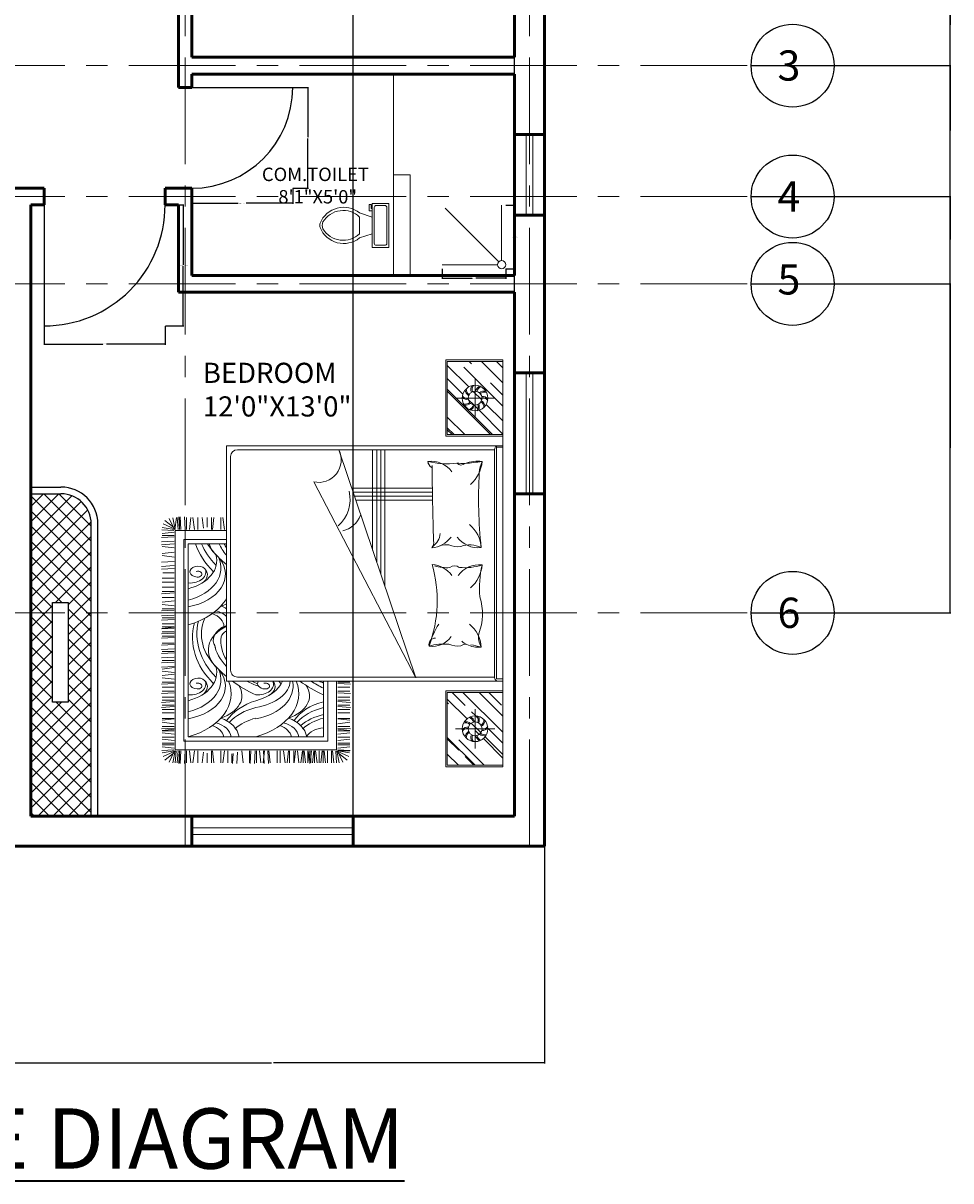
# Model space of a CAD drawing. Units: inches. Extents: x 10696 to 11614, y 5787 to 6498.
# Tile 7 of 9: x 11338 to 11614, y 5787 to 6132. Entities that reach past the tile are written whole.
import ezdxf

# ---------------------------------------------------------------- set-up
doc = ezdxf.new("R2010")
doc.units = ezdxf.units.IN
doc.linetypes.add('CENTER', pattern=[50.8, 31.75, -6.35, 6.35, -6.35])
for name, color, linetype, lineweight in [('A-ANNO-DIMS', 2, 'Continuous', 18), ('A-ANNO-TITL', 7, 'Continuous', 35), ('A-AREA-IDEN', 7, 'Continuous', 25), ('A-DOOR', 3, 'Continuous', 25), ('A-FLOR-CASE', 32, 'Continuous', 25), ('A-FLOR-CASE-PATT', 252, 'Continuous', 13), ('A-FLOR-FIXT', 9, 'Continuous', 20), ('A-FURN', 8, 'Continuous', 18), ('A-GLAZ', 4, 'Continuous', 20), ('A-GRID', 1, 'CENTER', 18), ('A-GRID-IDEN', 1, 'Continuous', 25), ('A-WALL', 7, 'Continuous', 50)]:
    doc.layers.add(name, color=color, linetype=linetype, lineweight=lineweight)
doc.styles.get("Standard").update_dxf_attribs({"font": 'arial.ttf'})
doc.dimstyles.get("Standard").update_dxf_attribs({"dimtxt": 0.18, "dimasz": 0.18, "dimexe": 0.18, "dimexo": 0.0625, "dimgap": 0.09, "dimtad": 0, "dimtih": 1, "dimtoh": 1, "dimdec": 4, "dimzin": 0, "dimdsep": 46, "dimtxsty": 'Standard', "dimcen": 0.09, "dimadec": 0, "dimazin": 0, "dimtfac": 1, "dimtdec": 4, "dimtofl": 0, "dimtmove": 0, "dimatfit": 3, "dimfxl": 1, "dimtolj": 1, "dimtzin": 0, "dimarcsym": 0})

# ---------------------------------------------------------------- blocks, each defined once
blk = doc.blocks.new('A$C64B41DC1')
for p, q in [((0, 2.5079), (2.9903, 2.5079)), ((0, 2.0879), (0, 2.5079)), ((0.012, 2.4618), (0.0581, 2.5079)), ((0.012, 2.3515), (0.1684, 2.5079)), ((0.012, 2.0999), (0.012, 2.5079)), ((0.0543, 2.2213), (0.3409, 2.5079)), ((0.1689, 2.4179), (0.2589, 2.5079)), ((0.3265, 2.386), (0.4484, 2.5079)), ((0.3699, 2.3332), (0.5445, 2.5079)), ((0.548, 2.5079), (0.548, 2.0999)), ((0.56, 2.5079), (0.56, 2.0879)), ((0.6301, 2.5079), (0.6301, 0.4779)), ((0.6401, 2.461), (0.6401, 2.5079)), ((0.6401, 2.5079), (2.344, 2.5079)), ((2.344, 2.5079), (2.3601, 2.5079)), ((2.344, 2.5079), (2.344, 2.461)), ((2.3601, 2.5079), (2.3601, 2.4761)), ((2.3601, 0.4779), (2.3601, 2.5079)), ((2.4303, 2.5079), (2.4303, 2.0879)), ((2.4423, 2.5079), (2.4423, 2.0999)), ((2.4423, 2.3333), (2.6169, 2.5079)), ((2.4423, 2.2145), (2.7357, 2.5079)), ((2.4423, 2.404), (2.5354, 2.4971)), ((2.705, 2.398), (2.8149, 2.5079)), ((2.7691, 2.3772), (2.8998, 2.5079)), ((2.7819, 2.3646), (2.9252, 2.5079)), ((2.9783, 2.0999), (2.9783, 2.5079)), ((2.9903, 2.0879), (2.9903, 2.5079)), ((0.2157, 2.0999), (0.548, 2.4322)), ((0.2299, 2.0999), (0.548, 2.418)), ((0.2804, 2.1597), (0.2804, 2.4481)), ((2.344, 2.461), (0.6401, 2.461)), ((0.6601, 2.4461), (1.4951, 2.4461)), ((0.6601, 2.4461), (0.6601, 0.5579)), ((1.4951, 2.4461), (0.6697, 2.4461)), ((2.3301, 2.4461), (1.4951, 2.4461)), ((2.3301, 0.5579), (2.3301, 2.4461)), ((2.7099, 2.1597), (2.7099, 2.4481)), ((0.1362, 2.3039), (0.4246, 2.3039)), ((0.2311, 2.2906), (0.2937, 2.3532)), ((0.3405, 2.3039), (0.3605, 2.3238)), ((2.8541, 2.3039), (2.5657, 2.3039)), ((2.5849, 2.2779), (2.6158, 2.3088)), ((2.6158, 2.3088), (2.6313, 2.3243)), ((2.6674, 2.2756), (2.7382, 2.3464)), ((2.7249, 2.3076), (2.7512, 2.3339)), ((2.7746, 2.0999), (2.9783, 2.3036)), ((2.7914, 2.1846), (2.9783, 2.3715)), ((0.012, 2.261), (0.0275, 2.2765)), ((0.0404, 2.0999), (0.1982, 2.2578)), ((0.1365, 2.0999), (0.251, 2.2144)), ((0.2905, 2.2539), (0.3304, 2.2938)), ((0.4194, 2.0999), (0.548, 2.2285)), ((2.4423, 2.1353), (2.5382, 2.2312)), ((2.4918, 2.0999), (2.6366, 2.2447)), ((2.9144, 2.2312), (2.9783, 2.2951)), ((0.4986, 2.0999), (0.548, 2.1493)), ((0.5127, 2.0999), (0.548, 2.1352)), ((2.7831, 2.0999), (2.8678, 2.1846)), ((2.8962, 2.0999), (2.9783, 2.182)), ((0.56, 2.0879), (0, 2.0879)), ((0.548, 2.0999), (0.012, 2.0999)), ((2.4303, 2.0879), (2.9903, 2.0879)), ((2.4423, 2.0999), (2.9783, 2.0999)), ((2.5172, 2.0999), (2.5269, 2.1096)), ((0.9415, 1.9902), (0.9415, 1.3975)), ((0.9715, 1.9906), (0.9715, 1.4076)), ((1.0015, 1.991), (1.0015, 1.4177)), ((1.0315, 1.9916), (1.0315, 1.4279)), ((2.3349, 1.8678), (0.6613, 1.3029)), ((0.8956, 1.1191), (2.3349, 1.8678)), ((1.6636, 1.6412), (0.6601, 1.6412)), ((1.5748, 1.6112), (0.6601, 1.6112)), ((2.3665, 1.295), (2.3665, 1.3839)), ((2.377, 1.295), (2.3822, 1.3891)), ((2.4032, 1.295), (2.4032, 1.3839)), ((2.4346, 1.295), (2.4346, 1.3839)), ((2.4451, 1.295), (2.4503, 1.3891)), ((2.4774, 1.2957), (2.4774, 1.3837)), ((2.5, 1.295), (2.5, 1.3839)), ((2.5105, 1.295), (2.5157, 1.3891)), ((2.5367, 1.295), (2.5367, 1.3839)), ((2.5471, 1.295), (2.5524, 1.3891)), ((2.5681, 1.295), (2.5681, 1.3839)), ((2.5918, 1.295), (2.5918, 1.3839)), ((2.6346, 1.2957), (2.6346, 1.3837)), ((2.6362, 1.2957), (2.6467, 1.3839)), ((2.6729, 1.295), (2.6624, 1.3839)), ((2.6938, 1.295), (2.6938, 1.3839)), ((2.7043, 1.295), (2.7095, 1.3891)), ((2.7127, 1.2957), (2.7232, 1.3839)), ((2.7253, 1.295), (2.7253, 1.3839)), ((2.7494, 1.295), (2.7389, 1.3839)), ((2.7718, 1.295), (2.7718, 1.3839)), ((2.7959, 1.295), (2.7854, 1.3839)), ((2.8146, 1.2957), (2.8146, 1.3837)), ((2.8146, 1.2957), (2.8146, 1.3837)), ((2.8282, 1.295), (2.8282, 1.3839)), ((2.8282, 1.295), (2.8282, 1.3839)), ((2.8523, 1.295), (2.8418, 1.3839)), ((2.8523, 1.295), (2.8418, 1.3839)), ((2.8653, 1.2966), (2.8688, 1.3861)), ((2.8711, 1.2957), (2.8711, 1.3837)), ((2.8711, 1.2957), (2.8875, 1.3822)), ((2.8765, 1.2958), (2.9132, 1.3758)), ((2.8893, 1.3011), (2.9394, 1.3636)), ((2.3601, 1.2873), (2.8639, 1.2873)), ((2.8639, 1.2873), (2.8639, 0.1018)), ((2.8713, 1.2927), (2.954, 1.3315)), ((2.8717, 1.2884), (2.9588, 1.3058)), ((2.8744, 1.2817), (2.9603, 1.2869)), ((2.3601, 1.2233), (2.7999, 1.2233)), ((2.3601, 1.1913), (2.7679, 1.1912)), ((2.7679, 1.1912), (2.7679, 0.1978)), ((2.7999, 1.2233), (2.7999, 0.1658)), ((2.8716, 1.2565), (2.9605, 1.2669)), ((2.8716, 1.2212), (2.9605, 1.2212)), ((2.8716, 1.1947), (2.9605, 1.2052)), ((2.8723, 1.2489), (2.9603, 1.2489)), ((2.8716, 1.181), (2.9605, 1.1705)), ((2.8716, 1.1595), (2.9605, 1.1595)), ((2.8716, 1.133), (2.9605, 1.1435)), ((2.8716, 1.1193), (2.9605, 1.1088)), ((2.8723, 1.1872), (2.9603, 1.1872)), ((2.8723, 1.1255), (2.9603, 1.1255)), ((2.8716, 1.1035), (2.9605, 1.093)), ((2.8716, 1.0965), (2.9605, 1.0965)), ((2.8716, 1.086), (2.9657, 1.0913)), ((2.8716, 1.0756), (2.9605, 1.0756)), ((2.8716, 1.0491), (2.9605, 1.0596)), ((2.8716, 1.0354), (2.9605, 1.0249)), ((2.8723, 1.0858), (2.9605, 1.0753)), ((2.8723, 1.0416), (2.9603, 1.0416)), ((2.8723, 0.9987), (2.9605, 1.0092)), ((2.8723, 0.985), (2.9605, 0.9745)), ((2.8723, 0.9735), (2.9603, 0.9735)), ((2.8723, 0.9408), (2.9603, 0.9408)), ((2.8716, 0.9346), (2.9605, 0.9241)), ((2.8723, 0.8979), (2.9605, 0.9084)), ((2.8723, 0.8726), (2.9603, 0.8726)), ((2.8716, 0.7885), (2.9605, 0.799)), ((2.8716, 0.7818), (2.9657, 0.787)), ((2.8723, 0.8505), (2.9603, 0.8505)), ((2.8716, 0.7503), (2.9657, 0.7556)), ((2.8716, 0.7204), (2.9605, 0.7309)), ((2.8716, 0.6995), (2.9605, 0.6995)), ((2.8716, 0.689), (2.9657, 0.6838)), ((2.8723, 0.7571), (2.9605, 0.7466)), ((2.8716, 0.6576), (2.9657, 0.6523)), ((2.8716, 0.6471), (2.9605, 0.6471)), ((2.8716, 0.5903), (2.9605, 0.6007)), ((2.882, 0.5582), (2.9657, 0.5536)), ((2.8909, 0.5263), (2.9657, 0.5222)), ((2.8928, 0.5169), (2.9605, 0.5169)), ((0.6301, 0.4779), (2.3601, 0.4779)), ((0.7101, 0.5079), (2.2801, 0.5079)), ((1.2465, 0.4625), (1.1576, 0.452)), ((1.2465, 0.4365), (1.1577, 0.4365)), ((1.2542, 0.1018), (1.2542, 0.4779)), ((1.3182, 0.1658), (1.3182, 0.4779)), ((1.3502, 0.1978), (1.3502, 0.4779)), ((2.8716, 0.4877), (2.9603, 0.4877)), ((2.8716, 0.4625), (2.9605, 0.452)), ((2.8716, 0.4365), (2.9603, 0.4365)), ((1.2465, 0.3746), (1.1576, 0.3851)), ((1.2465, 0.3684), (1.1577, 0.3684)), ((2.8716, 0.3746), (2.9605, 0.3851)), ((2.8716, 0.3684), (2.9603, 0.3684)), ((1.2355, 0.3092), (1.1576, 0.3)), ((1.2285, 0.3357), (1.1577, 0.3357)), ((1.2457, 0.2676), (1.1577, 0.2676)), ((2.8723, 0.2676), (2.9603, 0.2676)), ((2.8826, 0.3092), (2.9605, 0.3)), ((2.8896, 0.3357), (2.9603, 0.3357)), ((1.2465, 0.1742), (1.1524, 0.169)), ((1.2457, 0.2423), (1.1576, 0.2319)), ((1.2465, 0.2057), (1.1576, 0.2161)), ((1.2465, 0.1847), (1.1576, 0.1847)), ((2.7679, 0.1978), (1.3502, 0.1978)), ((2.8716, 0.2057), (2.9605, 0.2161)), ((2.8716, 0.1847), (2.9605, 0.1847)), ((2.8716, 0.1742), (2.9657, 0.169)), ((2.8723, 0.2423), (2.9605, 0.2319)), ((1.2465, 0.1428), (1.1524, 0.1376)), ((1.2465, 0.1334), (1.1524, 0.1281)), ((1.2465, 0.1323), (1.1576, 0.1323)), ((1.2465, 0.1323), (1.1576, 0.1323)), ((1.2465, 0.1), (1.1576, 0.1105)), ((1.2465, 0.1229), (1.1588, 0.1168)), ((1.2464, 0.1007), (1.1592, 0.0833)), ((1.2468, 0.0964), (1.1641, 0.0576)), ((1.2288, 0.088), (1.1787, 0.0255)), ((1.2415, 0.0933), (1.2049, 0.0133)), ((1.247, 0.0934), (1.2306, 0.0069)), ((1.2527, 0.0925), (1.2493, 0.003)), ((2.8639, 0.1018), (1.2542, 0.1018)), ((1.2658, 0.0941), (1.2762, 0.0052)), ((1.2899, 0.0941), (1.2899, 0.0052)), ((1.2999, 0.0941), (1.3051, 0)), ((2.7999, 0.1658), (1.3182, 0.1658)), ((1.3313, 0.0941), (1.3365, 0)), ((1.3523, 0.0941), (1.3575, 0)), ((1.3804, 0.0941), (1.3699, 0.0052)), ((1.4119, 0.0934), (1.4223, 0.0052)), ((1.4485, 0.0941), (1.438, 0.0052)), ((1.48, 0.0941), (1.4852, 0)), ((1.5114, 0.0941), (1.5166, 0)), ((1.5323, 0.0941), (1.5376, 0)), ((1.5638, 0.0941), (1.5638, 0.0105)), ((1.6021, 0.0941), (1.6021, 0.0052)), ((1.6336, 0.0941), (1.6336, 0.0052)), ((1.6702, 0.0941), (1.6702, 0.0052)), ((1.7017, 0.0941), (1.7017, 0.0052)), ((1.7122, 0.0941), (1.7174, 0)), ((1.7445, 0.0934), (1.7445, 0.0054)), ((1.7698, 0.0934), (1.7803, 0.0052)), ((1.8065, 0.0941), (1.796, 0.0052)), ((1.8274, 0.0941), (1.8274, 0.0052)), ((1.8379, 0.0941), (1.8431, 0)), ((1.8746, 0.0941), (1.8798, 0)), ((1.8955, 0.0941), (1.8955, 0.0052)), ((1.906, 0.0941), (1.9113, 0)), ((1.9384, 0.0934), (1.9384, 0.0054)), ((1.9609, 0.0941), (1.9609, 0.0052)), ((1.9636, 0.0934), (1.9741, 0.0052)), ((1.9714, 0.0941), (1.9766, 0)), ((1.9976, 0.0941), (1.9976, 0.0052)), ((2.0081, 0.0941), (2.0133, 0)), ((2.029, 0.0941), (2.029, 0.0052)), ((2.0395, 0.0941), (2.0447, 0)), ((2.0797, 0.0941), (2.0797, 0.0052)), ((2.0902, 0.0941), (2.0954, 0)), ((2.1216, 0.0941), (2.1269, 0)), ((2.1412, 0.0941), (2.1412, 0.0052)), ((2.1517, 0.0941), (2.1569, 0)), ((2.1831, 0.0941), (2.1884, 0)), ((2.2093, 0.0941), (2.2093, 0.0052)), ((2.2198, 0.0941), (2.225, 0)), ((2.2512, 0.0941), (2.2565, 0)), ((2.2603, 0.0934), (2.2707, 0.0052)), ((2.2969, 0.0941), (2.2864, 0.0052)), ((2.3089, 0.0934), (2.3193, 0.0052)), ((2.3455, 0.0941), (2.3351, 0.0052)), ((2.3665, 0.0941), (2.3665, 0.0052)), ((2.377, 0.0941), (2.3822, 0)), ((2.4032, 0.0941), (2.4032, 0.0052)), ((2.4346, 0.0941), (2.4346, 0.0052)), ((2.4451, 0.0941), (2.4503, 0)), ((2.4774, 0.0934), (2.4774, 0.0054)), ((2.5, 0.0941), (2.5, 0.0052)), ((2.5105, 0.0941), (2.5157, 0)), ((2.5367, 0.0941), (2.5367, 0.0052)), ((2.5471, 0.0941), (2.5524, 0)), ((2.5681, 0.0941), (2.5681, 0.0052)), ((2.5918, 0.0941), (2.5918, 0.0052)), ((2.6346, 0.0934), (2.6346, 0.0054)), ((2.6362, 0.0934), (2.6467, 0.0052)), ((2.6729, 0.0941), (2.6624, 0.0052)), ((2.6938, 0.0941), (2.6938, 0.0052)), ((2.7043, 0.0941), (2.7095, 0)), ((2.7127, 0.0934), (2.7232, 0.0052)), ((2.7253, 0.0941), (2.7253, 0.0052)), ((2.7494, 0.0941), (2.7389, 0.0052)), ((2.7718, 0.0941), (2.7718, 0.0052)), ((2.7959, 0.0941), (2.7854, 0.0052)), ((2.8146, 0.0934), (2.8146, 0.0054)), ((2.8282, 0.0941), (2.8282, 0.0052)), ((2.8523, 0.0941), (2.8418, 0.0052)), ((2.8653, 0.0925), (2.8688, 0.003)), ((2.8711, 0.0934), (2.8875, 0.0069)), ((2.8713, 0.0964), (2.954, 0.0576)), ((2.8716, 0.1428), (2.9657, 0.1376)), ((2.8716, 0.1334), (2.9657, 0.1281)), ((2.8716, 0.1323), (2.9605, 0.1323)), ((2.8716, 0.1229), (2.9593, 0.1168)), ((2.8717, 0.1007), (2.9588, 0.0833)), ((2.8744, 0.1074), (2.9603, 0.1022)), ((2.8765, 0.0933), (2.9132, 0.0133)), ((2.8893, 0.088), (2.9394, 0.0255))]:
    blk.add_line(p, q)
at = {"ltscale": 10}
for p, q in [((1.4859, 1.5812), (0.6601, 1.5812)), ((1.397, 1.5512), (0.6601, 1.5512))]:
    blk.add_line(p, q, dxfattribs=at)
for centre, radius in [((0.2804, 2.3039), 0.0942), ((2.7099, 2.3039), 0.0942), ((0.2804, 2.3039), 0.051), ((2.7099, 2.3039), 0.051)]:
    blk.add_circle(centre, radius)
for centre, radius, start, end in [((0.6601, 2.4761), 0.03, 180, 270), ((2.3301, 2.4761), 0.03, 270, 0), ((0.2887, 2.3745), 0.0605, 172.17003, 218.48975), ((0.2828, 2.3731), 0.0462, 160.30017, 220.53802), ((0.3286, 2.3561), 0.0605, 136.17003, 182.48975), ((0.3231, 2.3585), 0.0462, 124.30017, 184.53802), ((2.6672, 2.3585), 0.0462, 355.46198, 55.69983), ((2.6617, 2.3561), 0.0605, 357.51025, 43.82997), ((2.7075, 2.3731), 0.0462, 319.46198, 19.69983), ((2.7016, 2.3745), 0.0605, 321.51025, 7.82997), ((0.2457, 2.3659), 0.0605, 208.17003, 254.48975), ((0.2417, 2.3614), 0.0462, 196.30017, 256.53802), ((0.3501, 2.3178), 0.0605, 100.17003, 146.48975), ((0.347, 2.323), 0.0462, 88.30017, 148.53802), ((0.3449, 2.2742), 0.0605, 64.17003, 110.48975), ((0.3455, 2.2802), 0.0462, 52.30017, 112.53802), ((0.3151, 2.2419), 0.0605, 28.17003, 74.48975), ((1.0526, 2.3302), 0.3085, 175.30484, 198.69419), ((-0.8702, 2.0941), 1.6364, 4.80985, 9.18918), ((0.8579, 2.6278), 0.2948, 247.51785, 264.26696), ((0.728, 2.111), 0.245, 40.4189, 85.9871), ((1.0164, 5.7096), 3.3803, 266.81337, 276.16021), ((1.3963, 2.1044), 0.245, 94.0129, 139.5811), ((1.1858, 2.3288), 0.1943, 306.5711, 5.88998), ((1.5348, 2.2652), 0.1767, 151.77364, 201.69827), ((1.6986, 2.3355), 0.1943, 174.11002, 233.4289), ((1.1481, 2.2311), 0.3783, 353.49469, 19.18669), ((1.6871, 3.192), 0.8561, 257.74383, 273.62843), ((1.4882, 2.111), 0.245, 40.4189, 85.9871), ((1.8674, 1.9709), 0.3878, 68.20259, 108.9817), ((2.1269, 2.1044), 0.245, 94.0129, 139.5811), ((2.0342, 2.4856), 0.1563, 261.59582, 298.90918), ((1.9165, 2.3288), 0.1943, 333.73715, 5.88998), ((2.6058, 2.2028), 0.517, 163.60457, 172.3273), ((2.6448, 2.2802), 0.0462, 67.46198, 127.69983), ((2.6454, 2.2742), 0.0605, 69.51025, 115.82997), ((2.6752, 2.2419), 0.0605, 105.51025, 151.82997), ((2.6433, 2.323), 0.0462, 31.46198, 91.69983), ((2.6402, 2.3178), 0.0605, 33.51025, 79.82997), ((2.7486, 2.3614), 0.0462, 283.46198, 343.69983), ((2.7446, 2.3659), 0.0605, 285.51025, 331.82997), ((0.2153, 2.3276), 0.0462, 232.30017, 292.53802), ((0.2158, 2.3336), 0.0605, 244.17003, 290.48975), ((0.2138, 2.2848), 0.0462, 268.30017, 328.53802), ((0.2107, 2.29), 0.0605, 280.17003, 326.48975), ((0.2377, 2.2493), 0.0462, 304.30017, 4.53802), ((0.2322, 2.2517), 0.0605, 316.17003, 2.48975), ((0.2779, 2.2347), 0.0462, 340.30017, 40.53802), ((0.272, 2.2333), 0.0605, 352.17003, 38.48975), ((0.3191, 2.2464), 0.0462, 16.30017, 76.53802), ((0.7274, 2.2013), 0.0446, 314.4736, 42.17134), ((-1.6008, 2.277), 2.3618, 357.39054, 358.88764), ((1.9165, 2.3288), 0.1943, 320.94042, 333.73715), ((2.1347, 2.2313), 0.0459, 165.35061, 223.26844), ((2.6712, 2.2464), 0.0462, 103.46198, 163.69983), ((2.7182, 2.2333), 0.0605, 141.51025, 187.82997), ((2.7123, 2.2347), 0.0462, 139.46198, 199.69983), ((2.7581, 2.2517), 0.0605, 177.51025, 223.82997), ((2.7526, 2.2493), 0.0462, 175.46198, 235.69983), ((2.7796, 2.29), 0.0605, 213.51025, 259.82997), ((2.7765, 2.2848), 0.0462, 211.46198, 271.69983), ((2.7744, 2.3336), 0.0605, 249.51025, 295.82997), ((2.775, 2.3276), 0.0462, 247.46198, 307.69983), ((0.9385, 1.978), 0.1943, 126.5711, 185.88998), ((0.2688, 2.0945), 0.4956, 344.0243, 8.70709), ((1.1858, 1.9714), 0.1943, 4.31813, 53.4289), ((1.204, 2.1778), 0.1681, 337.01697, 7.53676), ((1.7059, 1.9714), 0.204, 127.11975, 175.09005), ((1.5671, 2.1546), 0.0547, 142.08329, 220.902), ((1.9394, 1.991), 0.1651, 351.26213, 55.75721), ((1.9346, 2.1778), 0.1681, 337.01697, 7.53676), ((1.2687, 1.9248), 0.1223, 33.62799, 86.47438), ((1.5415, 2.0969), 0.1834, 175.22328, 196.23004), ((1.1965, 2.0983), 0.3299, 343.79543, 3.55541), ((2.4617, 2.0719), 0.3745, 173.82958, 196.4356), ((0.7417, 2.0149), 0.057, 273.47085, 328.54118), ((0.728, 2.2025), 0.245, 274.0129, 278.34166), ((0.7246, 18.8439), 16.8552, 270.17399, 272.05214), ((1.3401, 1.9404), 0.0603, 49.09906, 101.37023), ((1.7676, 1.0629), 0.9631, 69.65065, 105.96307), ((2.2748, 2.5795), 0.6373, 238.34989, 254.31375), ((2.0911, 2.0123), 0.0478, 179.77267, 283.80184), ((1.0747, 1.2871), 0.1871, 14.1863, 69.12121), ((1.0274, 1.1334), 0.2527, 40.62904, 104.37123), ((0.7347, 1.1553), 0.1649, 347.31088, 116.44537), ((0.7101, 0.5579), 0.05, 180, 270), ((2.2801, 0.5579), 0.05, 270, 0)]:
    blk.add_arc(centre, radius, start, end)
for centre, major_axis, ratio, start_param, end_param in [((1.9938, 1.6262), (0, -0.7531), 0.68, 0.797284, 0.954936), ((2.0643, 1.466), (0, -0.5322), 0.68, 7.239912, 7.311536), ((1.9052, 1.7397), (0, -0.9842), 0.68, 0.74745, 0.979724), ((2.7455, 1.3081), (0, 0.3614), 0.68, 1.900046, 2.742661), ((2.7868, 1.3081), (0, 0.3614), 0.68, 1.900046, 2.614747), ((2.8372, 1.3081), (0, 0.3614), 0.68, 1.900046, 2.479658), ((2.8607, 1.3211), (0, 0.3614), 0.68, 1.938265, 2.479658), ((2.8057, 1.2079), (0, -0.1524), 0.68, 4.821745, 5.895886), ((2.4665, 0.8216), (0, -0.2664), 0.68, 2.006169, 3.565187), ((2.4513, 0.5069), (0, 0.502), 0.68, 5.095327, 6.553458), ((2.7862, 0.8069), (0, -0.2615), 0.68, 3.244645, 4.205018), ((2.396, 0.6032), (0, 0.3641), 0.68, -1.3172, 0.145284), ((2.3507, 0.5642), (0.0073, 0.3819), 0.56205, -1.21172, -0.009991), ((2.7784, 0.8289), (0, -0.1802), 0.68, 3.227058, 4.318474), ((2.7821, 0.7971), (0, -0.1589), 0.68, 3.272942, 4.229533), ((2.2964, 0.5771), (0, -0.3263), 0.68, 1.938944, 2.850232), ((2.0403, 1.6015), (0, -0.8763), 0.68, 6.849801, 6.887077), ((2.4005, 0.7132), (0, -0.1214), 0.68, 2.284368, 3.652258), ((2.3834, 0.7081), (0, 0.1147), 0.68, 4.593909, 6.585576), ((2.3961, 0.7628), (0, -0.0317), 0.68, 1.462497, 5.046281), ((2.3774, 0.7653), (0, -0.0593), 0.68, 5.841311, 7.755362), ((1.9938, 1.1295), (-0.0678, 0.7439), 0.610498, 3.917146, 4.063997), ((2.0643, 0.9693), (0, -0.5322), 0.68, 7.239912, 7.336618), ((1.9052, 1.243), (0, -0.9842), 0.68, 0.74745, 0.979724), ((2.7455, 0.8114), (-0.0599, 0.3735), 0.695517, 1.775813, 2.548612), ((2.7868, 0.8114), (0, 0.3614), 0.68, 1.900046, 2.614747), ((2.8607, 0.8243), (0, 0.3614), 0.68, 1.938265, 2.479658), ((2.4665, 0.3249), (0, -0.2664), 0.68, 2.006169, 3.565187), ((2.4513, 0.0102), (0, 0.502), 0.68, 5.095327, 6.553458), ((2.7862, 0.3102), (0, -0.2615), 0.68, 3.244645, 4.205018), ((2.7784, 0.3322), (0, -0.1802), 0.68, 3.227058, 4.318474), ((1.242, 0.9693), (0, -0.5322), 0.68, 6.586764, 6.677612), ((1.1714, 1.1295), (-0.1157, 0.7241), 0.59432, 3.291697, 3.50733), ((1.474, 0.0804), (0, -0.3263), 0.68, 1.938944, 3.339184), ((1.0828, 1.243), (0, -0.9842), 0.68, 0.565948, 0.680366), ((1.5283, 0.0674), (0, -0.3703), 0.68, 1.930561, 3.464283), ((1.5736, 0.1065), (0, 0.3641), 0.68, -1.3172, 0.476403), ((1.6289, 0.0102), (0, 0.502), 0.68, 6.655152, 6.661293), ((1.6289, 0.0102), (0, 0.502), 0.68, 5.095327, 5.911219), ((1.6442, 0.3249), (0, -0.2664), 0.68, 2.006169, 2.182797), ((1.9638, 0.3102), (0, -0.2615), 0.68, 4.015924, 4.205018), ((1.956, 0.3322), (0, -0.1802), 0.68, 3.770744, 4.318474), ((1.9597, 0.3004), (0, -0.1589), 0.68, 3.14258, 4.229533), ((2.0606, 0.5616), (0, -0.1803), 0.68, 5.194792, 5.929328), ((2.0606, 0.5616), (0, -0.1803), 0.68, 5.194792, 6.723255), ((2.1315, 0.6603), (0, -0.3155), 0.68, 5.328638, 6.949396), ((2.0549, 0.5656), (0, -0.1303), 0.68, 5.450951, 6.054641), ((2.0643, 0.9693), (0, -0.5322), 0.68, 6.20013, 6.677612), ((1.9938, 1.1295), (-0.0678, 0.7439), 0.610498, 3.199135, 3.592282), ((2.2964, 0.0804), (0, -0.3263), 0.68, 1.938944, 3.339184), ((1.9052, 1.243), (0, -0.9842), 0.68, 0.565948, 0.680366), ((2.3507, 0.0674), (0, -0.3703), 0.68, 1.930561, 3.464283), ((2.396, 0.1065), (0, 0.3641), 0.68, -1.3172, 0.476403), ((2.4513, 0.0102), (0, 0.502), 0.68, 6.655152, 6.661293), ((2.7821, 0.3004), (0, -0.1589), 0.68, 3.272942, 4.229533), ((1.1933, 0.9181), (0, -0.624), 0.68, 0.378672, 0.625379), ((1.3091, 0.6603), (0, -0.3155), 0.68, 6.475719, 6.949396), ((1.1911, 1.1066), (0, 0.8458), 0.68, 3.421828, 3.728616), ((1.2179, 1.1047), (0, -0.8763), 0.68, 6.507006, 6.887077), ((1.5781, 0.2165), (0, -0.1214), 0.68, 2.284368, 3.726131), ((2.0157, 0.9181), (0, -0.624), 0.68, -0.280078, 0.625379), ((2.0135, 1.1066), (0, 0.8458), 0.68, 2.978727, 3.728616), ((2.0403, 1.1047), (0, -0.8763), 0.68, 6.099302, 6.887077), ((2.4005, 0.2165), (0, -0.1214), 0.68, 2.284368, 3.726131), ((1.555, 0.2685), (0, -0.0593), 0.68, 3.732151, 7.755362), ((1.561, 0.2114), (0, 0.1147), 0.68, 4.593909, 6.647252), ((1.5737, 0.2661), (0, -0.0317), 0.68, 1.462497, 5.046281), ((2.3774, 0.2685), (0, -0.0593), 0.68, 3.732151, 7.755362), ((2.3834, 0.2114), (0, 0.1147), 0.68, 4.593909, 6.647252), ((2.3961, 0.2661), (0, -0.0317), 0.68, 1.462497, 5.046281)]:
    blk.add_ellipse(centre, major_axis=major_axis, ratio=ratio, start_param=start_param, end_param=end_param)
blk = doc.blocks.new('*U10')
for p, q in [((9.5, -6), (9.5, -2)), ((-10, -8.5), (-8, -8.5)), ((-10, -9.5), (-10, -8.5)), ((-7, -9.5), (-10, -9.5)), ((-8, -8.5), (-8, -8)), ((-7, -8), (-7, -9.5)), ((-4, -8), (-6, -14)), ((4, -8), (6, -14)), ((4, -14), (-4, -14))]:
    blk.add_line(p, q)
blk.add_lwpolyline([(10.5, -8), (10.5, 0), (-10.5, 0), (-10.5, -8)], close=True)
for points in [[(-9.5, -2), (-9.5, -6)], [(8.5, -1), (-8.5, -1)], [(-8.5, -7), (8.5, -7)]]:
    blk.add_lwpolyline(points)
for centre, radius, start, end in [((-8.62, -1.88), 0.884, 81.8699, 188.1301), ((8.62, -1.88), 0.884, 351.8699, 98.1301), ((-8.62, -6.12), 0.884, 171.8699, 278.1301), ((8.62, -6.12), 0.884, 261.8699, 8.1301), ((3.52, -21.58), 12.17, 141.4691, 247.9714), ((4.2, -21.82), 11.33, 136.3677, 238.9468), ((-3.52, -21.58), 12.17, 292.0284, 38.5307), ((-4.2, -21.82), 11.33, 301.053, 43.6321), ((0, -27.88), 4, 245.7318, 294.2682), ((0, -29), 4, 254.8605, 285.1395)]:
    blk.add_arc(centre, radius, start, end)
blk = doc.blocks.new('DOOR-SINGLE-30')
blk.add_line((0, 30), (30, 30))
blk.add_arc((0, 30), 30, 270, 0)
blk = doc.blocks.new('DOOR-SINGLE-36-BEDROOM')
blk.add_line((0, 36), (0, 0))
blk.add_arc((0.1, 35.9), 35.9, 269.8411, 0.1589)
blk = doc.blocks.new('WIN-GLAZ-24')
for p, q in [((0, 24), (0, 0)), ((2, 24), (2, 0))]:
    blk.add_line(p, q)
blk = doc.blocks.new('WIN-GLAZ-36')
for p, q in [((0, 0), (0, 36)), ((2, 0), (2, 36))]:
    blk.add_line(p, q)
blk = doc.blocks.new('WIN-GLAZ-48')
for p, q in [((0, 48), (0, 0)), ((2, 48), (2, 0))]:
    blk.add_line(p, q)
blk = doc.blocks.new('SHOWER-SCREEN')
for p, q in [((0, 0), (0, 60)), ((0, 30), (5, 30)), ((5, 0), (5, 30))]:
    blk.add_line(p, q)
blk = doc.blocks.new('SHOWER-DRAIN')
for p, q in [((16.81, 2.05), (0.86, 18)), ((17.68, 2.42), (17.68, 18.95)), ((16.47, 1.21), (0, 1.21))]:
    blk.add_line(p, q)
blk.add_circle((17.68, 1.21), 1.21)
blk = doc.blocks.new('*D44')
at = {"layer": 'A-ANNO-DIMS', "color": 0, "lineweight": -2, "transparency": 16777216}
for p, q in [((11387.77, 6083.01), (11387.77, 6078.39)), ((11417.77, 6083.01), (11417.77, 6078.39)), ((11387.95, 6078.57), (11401.58, 6078.57)), ((11417.59, 6078.57), (11403.96, 6078.57))]:
    blk.add_line(p, q, dxfattribs=at)
at = {"layer": 'A-ANNO-DIMS', "color": 0, "transparency": 16777216}
for points in [[(11387.95, 6078.6), (11387.95, 6078.54), (11387.77, 6078.57)], [(11417.59, 6078.6), (11417.59, 6078.54), (11417.77, 6078.57)]]:
    blk.add_solid(points, dxfattribs=at)
at = {"layer": 'Defpoints', "color": 0, "transparency": 16777216}
for p in [(11387.77, 6083.07), (11417.77, 6083.07), (11417.77, 6078.57)]:
    blk.add_point(p, dxfattribs=at)
at = {"layer": 'A-ANNO-DIMS', "color": 0, "transparency": 16777216, "insert": (11402.77, 6078.57), "char_height": 0.18, "attachment_point": 5}
blk.add_mtext('\\A1;WC DOOR 30 TYP.', dxfattribs=at)
blk = doc.blocks.new('*D45')
at = {"layer": 'A-ANNO-DIMS', "color": 0, "lineweight": -2, "transparency": 16777216}
for p, q in [((11417.83, 6113.07), (11422.45, 6113.07)), ((11422.27, 6112.89), (11422.27, 6098.25)), ((11422.27, 6083.25), (11422.27, 6097.89)), ((11417.83, 6083.07), (11422.45, 6083.07))]:
    blk.add_line(p, q, dxfattribs=at)
at = {"layer": 'A-ANNO-DIMS', "color": 0, "transparency": 16777216}
for points in [[(11422.24, 6112.89), (11422.3, 6112.89), (11422.27, 6113.07)], [(11422.24, 6083.25), (11422.3, 6083.25), (11422.27, 6083.07)]]:
    blk.add_solid(points, dxfattribs=at)
at = {"layer": 'Defpoints', "color": 0, "transparency": 16777216}
for p in [(11417.77, 6113.07), (11422.27, 6113.07), (11417.77, 6083.07)]:
    blk.add_point(p, dxfattribs=at)
at = {"layer": 'A-ANNO-DIMS', "color": 0, "transparency": 16777216, "insert": (11422.27, 6098.07), "char_height": 0.18, "attachment_point": 5}
blk.add_mtext('\\A1;30 TYP.', dxfattribs=at)
blk = doc.blocks.new('*D46')
at = {"layer": 'A-ANNO-DIMS', "color": 0, "lineweight": -2, "transparency": 16777216}
for p, q in [((11379.86, 6078.07), (11385.38, 6078.07)), ((11385.2, 6077.89), (11385.2, 6060.24)), ((11385.2, 6042.22), (11385.2, 6059.87)), ((11379.86, 6042.04), (11385.38, 6042.04))]:
    blk.add_line(p, q, dxfattribs=at)
at = {"layer": 'A-ANNO-DIMS', "color": 0, "transparency": 16777216}
for points in [[(11385.17, 6077.89), (11385.23, 6077.89), (11385.2, 6078.07)], [(11385.17, 6042.22), (11385.23, 6042.22), (11385.2, 6042.04)]]:
    blk.add_solid(points, dxfattribs=at)
at = {"layer": 'Defpoints', "color": 0, "transparency": 16777216}
for p in [(11379.79, 6078.07), (11385.2, 6078.07), (11379.79, 6042.04)]:
    blk.add_point(p, dxfattribs=at)
at = {"layer": 'A-ANNO-DIMS', "color": 0, "transparency": 16777216, "insert": (11385.2, 6060.06), "char_height": 0.18, "attachment_point": 5}
blk.add_mtext('\\A1;BEDROOM DOOR 36 TYP.', dxfattribs=at)
blk = doc.blocks.new('*D47')
at = {"layer": 'A-ANNO-DIMS', "color": 0, "lineweight": -2, "transparency": 16777216}
for p, q in [((11343.77, 6041.98), (11343.77, 6036.46)), ((11379.79, 6041.98), (11379.79, 6036.46)), ((11343.95, 6036.64), (11361.25, 6036.64)), ((11379.61, 6036.64), (11362.31, 6036.64))]:
    blk.add_line(p, q, dxfattribs=at)
at = {"layer": 'A-ANNO-DIMS', "color": 0, "transparency": 16777216}
for points in [[(11343.95, 6036.67), (11343.95, 6036.61), (11343.77, 6036.64)], [(11379.61, 6036.67), (11379.61, 6036.61), (11379.79, 6036.64)]]:
    blk.add_solid(points, dxfattribs=at)
at = {"layer": 'Defpoints', "color": 0, "transparency": 16777216}
for p in [(11343.77, 6042.04), (11379.79, 6042.04), (11379.79, 6036.64)]:
    blk.add_point(p, dxfattribs=at)
at = {"layer": 'A-ANNO-DIMS', "color": 0, "transparency": 16777216, "insert": (11361.78, 6036.64), "char_height": 0.18, "attachment_point": 5}
blk.add_mtext('\\A1;36 TYP.', dxfattribs=at)
blk = doc.blocks.new('*D62')
at = {"layer": 'A-ANNO-DIMS', "color": 0, "lineweight": -2, "transparency": 16777216}
for p, q in [((11481.25, 6078.02), (11484.21, 6078.02)), ((11484.03, 6077.84), (11484.03, 6068.73)), ((11484.03, 6059.25), (11484.03, 6068.37)), ((11481.25, 6059.07), (11484.21, 6059.07))]:
    blk.add_line(p, q, dxfattribs=at)
at = {"layer": 'A-ANNO-DIMS', "color": 0, "transparency": 16777216}
for points in [[(11484, 6077.84), (11484.06, 6077.84), (11484.03, 6078.02)], [(11484, 6059.25), (11484.06, 6059.25), (11484.03, 6059.07)]]:
    blk.add_solid(points, dxfattribs=at)
at = {"layer": 'Defpoints', "color": 0, "transparency": 16777216}
for p in [(11481.19, 6078.02), (11484.03, 6078.02), (11481.19, 6059.07)]:
    blk.add_point(p, dxfattribs=at)
at = {"layer": 'A-ANNO-DIMS', "color": 0, "transparency": 16777216, "insert": (11484.03, 6068.55), "char_height": 0.18, "attachment_point": 5}
blk.add_mtext('\\A1;DRAIN 19 TYP.', dxfattribs=at)
blk = doc.blocks.new('*D63')
at = {"layer": 'A-ANNO-DIMS', "color": 0, "lineweight": -2, "transparency": 16777216}
for p, q in [((11462.3, 6059.01), (11462.3, 6056.05)), ((11481.19, 6059.01), (11481.19, 6056.05)), ((11462.48, 6056.23), (11471.23, 6056.23)), ((11481.01, 6056.23), (11472.26, 6056.23))]:
    blk.add_line(p, q, dxfattribs=at)
at = {"layer": 'A-ANNO-DIMS', "color": 0, "transparency": 16777216}
for points in [[(11462.48, 6056.26), (11462.48, 6056.2), (11462.3, 6056.23)], [(11481.01, 6056.26), (11481.01, 6056.2), (11481.19, 6056.23)]]:
    blk.add_solid(points, dxfattribs=at)
at = {"layer": 'Defpoints', "color": 0, "transparency": 16777216}
for p in [(11462.3, 6059.07), (11481.19, 6059.07), (11481.19, 6056.23)]:
    blk.add_point(p, dxfattribs=at)
at = {"layer": 'A-ANNO-DIMS', "color": 0, "transparency": 16777216, "insert": (11471.75, 6056.23), "char_height": 0.18, "attachment_point": 5}
blk.add_mtext('\\A1;19 TYP.', dxfattribs=at)
blk = doc.blocks.new('*D76')
at = {"layer": 'A-ANNO-DIMS', "color": 0, "lineweight": -2, "transparency": 16777216}
for p, q in [((11330.77, 5887.01), (11330.77, 5822.34)), ((11492.77, 5887.01), (11492.77, 5822.34)), ((11330.95, 5822.52), (11411.49, 5822.52)), ((11492.59, 5822.52), (11412.05, 5822.52))]:
    blk.add_line(p, q, dxfattribs=at)
at = {"layer": 'A-ANNO-DIMS', "color": 0, "transparency": 16777216}
for points in [[(11330.95, 5822.55), (11330.95, 5822.49), (11330.77, 5822.52)], [(11492.59, 5822.55), (11492.59, 5822.49), (11492.77, 5822.52)]]:
    blk.add_solid(points, dxfattribs=at)
at = {"layer": 'Defpoints', "color": 0, "transparency": 16777216}
for p in [(11330.77, 5887.07), (11492.77, 5887.07), (11492.77, 5822.52)]:
    blk.add_point(p, dxfattribs=at)
at = {"layer": 'A-ANNO-DIMS', "color": 0, "transparency": 16777216, "insert": (11411.77, 5822.52), "char_height": 0.18, "attachment_point": 5}
blk.add_mtext('\\A1;162', dxfattribs=at)
blk = doc.blocks.new('*D82')
at = {"layer": 'A-ANNO-DIMS', "color": 0, "lineweight": -2, "transparency": 16777216}
for p, q in [((11554.32, 6184.57), (11613.7, 6184.57)), ((11613.52, 6184.39), (11613.52, 6152.25)), ((11613.52, 6119.75), (11613.52, 6151.89)), ((11554.32, 6119.57), (11613.7, 6119.57))]:
    blk.add_line(p, q, dxfattribs=at)
at = {"layer": 'A-ANNO-DIMS', "color": 0, "transparency": 16777216}
for points in [[(11613.49, 6184.39), (11613.55, 6184.39), (11613.52, 6184.57)], [(11613.49, 6119.75), (11613.55, 6119.75), (11613.52, 6119.57)]]:
    blk.add_solid(points, dxfattribs=at)
at = {"layer": 'Defpoints', "color": 0, "transparency": 16777216}
for p in [(11554.26, 6184.57), (11554.26, 6119.57), (11613.52, 6119.57)]:
    blk.add_point(p, dxfattribs=at)
at = {"layer": 'A-ANNO-DIMS', "color": 0, "transparency": 16777216, "insert": (11613.52, 6152.07), "char_height": 0.18, "attachment_point": 5}
blk.add_mtext('\\A1;65', dxfattribs=at)
blk = doc.blocks.new('*D83')
at = {"layer": 'A-ANNO-DIMS', "color": 0, "lineweight": -2, "transparency": 16777216}
for p, q in [((11554.32, 6119.57), (11613.7, 6119.57)), ((11613.52, 6119.39), (11613.52, 6100.25)), ((11613.52, 6080.75), (11613.52, 6099.89)), ((11554.32, 6080.57), (11613.7, 6080.57))]:
    blk.add_line(p, q, dxfattribs=at)
at = {"layer": 'A-ANNO-DIMS', "color": 0, "transparency": 16777216}
for points in [[(11613.49, 6119.39), (11613.55, 6119.39), (11613.52, 6119.57)], [(11613.49, 6080.75), (11613.55, 6080.75), (11613.52, 6080.57)]]:
    blk.add_solid(points, dxfattribs=at)
at = {"layer": 'Defpoints', "color": 0, "transparency": 16777216}
for p in [(11554.26, 6119.57), (11554.26, 6080.57), (11613.52, 6080.57)]:
    blk.add_point(p, dxfattribs=at)
at = {"layer": 'A-ANNO-DIMS', "color": 0, "transparency": 16777216, "insert": (11613.52, 6100.07), "char_height": 0.18, "attachment_point": 5}
blk.add_mtext('\\A1;39', dxfattribs=at)
blk = doc.blocks.new('*D84')
at = {"layer": 'A-ANNO-DIMS', "color": 0, "lineweight": -2, "transparency": 16777216}
for p, q in [((11554.32, 6080.57), (11613.7, 6080.57)), ((11613.52, 6080.39), (11613.52, 6067.75)), ((11613.52, 6054.75), (11613.52, 6067.39)), ((11554.32, 6054.57), (11613.7, 6054.57))]:
    blk.add_line(p, q, dxfattribs=at)
at = {"layer": 'A-ANNO-DIMS', "color": 0, "transparency": 16777216}
for points in [[(11613.49, 6080.39), (11613.55, 6080.39), (11613.52, 6080.57)], [(11613.49, 6054.75), (11613.55, 6054.75), (11613.52, 6054.57)]]:
    blk.add_solid(points, dxfattribs=at)
at = {"layer": 'Defpoints', "color": 0, "transparency": 16777216}
for p in [(11554.26, 6080.57), (11554.26, 6054.57), (11613.52, 6054.57)]:
    blk.add_point(p, dxfattribs=at)
at = {"layer": 'A-ANNO-DIMS', "color": 0, "transparency": 16777216, "insert": (11613.52, 6067.57), "char_height": 0.18, "attachment_point": 5}
blk.add_mtext('\\A1;26', dxfattribs=at)
blk = doc.blocks.new('*D85')
at = {"layer": 'A-ANNO-DIMS', "color": 0, "lineweight": -2, "transparency": 16777216}
for p, q in [((11554.32, 6054.57), (11613.7, 6054.57)), ((11613.52, 6054.39), (11613.52, 6005.75)), ((11613.52, 5956.75), (11613.52, 6005.39)), ((11554.32, 5956.57), (11613.7, 5956.57))]:
    blk.add_line(p, q, dxfattribs=at)
at = {"layer": 'A-ANNO-DIMS', "color": 0, "transparency": 16777216}
for points in [[(11613.49, 6054.39), (11613.55, 6054.39), (11613.52, 6054.57)], [(11613.49, 5956.75), (11613.55, 5956.75), (11613.52, 5956.57)]]:
    blk.add_solid(points, dxfattribs=at)
at = {"layer": 'Defpoints', "color": 0, "transparency": 16777216}
for p in [(11554.26, 6054.57), (11554.26, 5956.57), (11613.52, 5956.57)]:
    blk.add_point(p, dxfattribs=at)
at = {"layer": 'A-ANNO-DIMS', "color": 0, "transparency": 16777216, "insert": (11613.52, 6005.57), "char_height": 0.18, "attachment_point": 5}
blk.add_mtext('\\A1;98', dxfattribs=at)
blk = doc.blocks.new('*D86')
at = {"layer": 'A-ANNO-DIMS', "color": 0, "lineweight": -2, "transparency": 16777216}
for p, q in [((11579.03, 6306.57), (11613.7, 6306.57)), ((11613.52, 6306.39), (11613.52, 6131.75)), ((11613.52, 5956.75), (11613.52, 6131.39)), ((11579.03, 5956.57), (11613.7, 5956.57))]:
    blk.add_line(p, q, dxfattribs=at)
at = {"layer": 'A-ANNO-DIMS', "color": 0, "transparency": 16777216}
for points in [[(11613.49, 6306.39), (11613.55, 6306.39), (11613.52, 6306.57)], [(11613.49, 5956.75), (11613.55, 5956.75), (11613.52, 5956.57)]]:
    blk.add_solid(points, dxfattribs=at)
at = {"layer": 'Defpoints', "color": 0, "transparency": 16777216}
for p in [(11578.97, 6306.57), (11578.97, 5956.57), (11613.52, 5956.57)]:
    blk.add_point(p, dxfattribs=at)
at = {"layer": 'A-ANNO-DIMS', "color": 0, "transparency": 16777216, "insert": (11613.52, 6131.57), "char_height": 0.18, "attachment_point": 5}
blk.add_mtext('\\A1;350', dxfattribs=at)
blk = doc.blocks.new('*D94')
at = {"layer": 'A-ANNO-DIMS', "color": 0, "lineweight": -2, "transparency": 16777216}
for p, q in [((11435.77, 5896.13), (11435.77, 6497.62)), ((11435.95, 6497.44), (11459.54, 6497.44)), ((11483.59, 6497.44), (11459.99, 6497.44)), ((11483.77, 5896.13), (11483.77, 6497.62))]:
    blk.add_line(p, q, dxfattribs=at)
at = {"layer": 'A-ANNO-DIMS', "color": 0, "transparency": 16777216}
for points in [[(11435.95, 6497.47), (11435.95, 6497.41), (11435.77, 6497.44)], [(11483.59, 6497.47), (11483.59, 6497.41), (11483.77, 6497.44)]]:
    blk.add_solid(points, dxfattribs=at)
at = {"layer": 'Defpoints', "color": 0, "transparency": 16777216}
for p in [(11435.77, 6497.44), (11435.77, 5896.07), (11483.77, 5896.07)]:
    blk.add_point(p, dxfattribs=at)
at = {"layer": 'A-ANNO-DIMS', "color": 0, "transparency": 16777216, "insert": (11459.77, 6497.44), "char_height": 0.18, "attachment_point": 5}
blk.add_mtext('\\A1;48', dxfattribs=at)

msp = doc.modelspace()

# ---------------------------------------------------------------- hatches: boundary and pattern name
at = {"layer": 'A-FLOR-CASE-PATT'}
h = msp.add_hatch(dxfattribs=at)
h.set_pattern_fill('ANSI37', color=256)
h.set_pattern_definition([(45, (434.8545, 0), (-2.245064, 2.245064), []), (135, (434.8545, 0), (-2.245064, -2.245064), [])])
h.paths.add_polyline_path([(11357.767, 5983.07, 0.4142136), (11348.767, 5992.07), (11339.767, 5992.07), (11339.767, 5896.07), (11357.767, 5896.07)])
h.paths.add_polyline_path([(11350.964, 5930.013), (11346.215, 5930.013), (11346.215, 5959.701), (11350.964, 5959.701)], flags=16)

# ---------------------------------------------------------------- linework, layer by layer
at = {"layer": 'A-FLOR-CASE'}
for p, q in [((11339.767, 5994.07), (11348.767, 5994.07)), ((11339.767, 5992.07), (11348.767, 5992.07)), ((11357.767, 5896.07), (11357.767, 5983.07)), ((11359.767, 5896.07), (11359.767, 5983.07))]:
    msp.add_line(p, q, dxfattribs=at)
msp.add_lwpolyline([(11346.215, 5959.701), (11350.964, 5959.701), (11350.964, 5930.013), (11346.215, 5930.013)], close=True, dxfattribs=at)
for radius in [11, 9]:
    msp.add_arc((11348.767, 5983.07), radius, 0, 90, dxfattribs=at)
at = {"layer": 'A-GRID'}
for p, q in [((11385.767, 5887.07), (11385.767, 6426.679)), ((11488.267, 5887.07), (11488.267, 6426.679)), ((11165.767, 6119.57), (11554.26, 6119.57)), ((11165.767, 6080.57), (11554.26, 6080.57)), ((11165.767, 6054.57), (11554.26, 6054.57)), ((11165.767, 5956.57), (11554.26, 5956.57))]:
    msp.add_line(p, q, dxfattribs=at)
at = {"layer": 'A-GRID-IDEN'}
for centre in [(11566.613, 6119.57), (11566.613, 6080.57), (11566.613, 6054.57), (11566.613, 5956.57)]:
    msp.add_circle(centre, 12.353, dxfattribs=at)
at = {"layer": 'A-WALL'}
for p, q in [((11492.767, 5887.07), (11492.767, 6311.07)), ((11387.767, 6122.07), (11387.767, 6187.07)), ((11383.767, 6113.07), (11383.767, 6182.07)), ((11483.767, 6122.07), (11483.767, 6182.07)), ((11387.767, 6122.07), (11483.767, 6122.07)), ((11387.767, 6117.07), (11483.767, 6117.07)), ((11387.767, 6113.07), (11387.767, 6117.07)), ((11483.767, 6057.07), (11483.767, 6117.07)), ((11383.767, 6113.07), (11387.767, 6113.07)), ((11483.767, 6099.07), (11492.767, 6099.07)), ((11334.767, 6083.07), (11343.767, 6083.07)), ((11343.767, 6078.07), (11343.767, 6083.07)), ((11379.767, 6083.07), (11387.767, 6083.07)), ((11379.767, 6078.07), (11379.767, 6083.07)), ((11387.767, 6057.07), (11387.767, 6083.07)), ((11339.767, 6078.07), (11343.767, 6078.07)), ((11339.767, 5896.07), (11339.767, 6078.07)), ((11379.767, 6078.07), (11383.767, 6078.07)), ((11383.767, 6052.07), (11383.767, 6078.07)), ((11483.767, 6075.07), (11492.767, 6075.07)), ((11387.767, 6057.07), (11483.767, 6057.07)), ((11383.767, 6052.07), (11483.767, 6052.07)), ((11483.767, 5896.07), (11483.767, 6052.07)), ((11483.767, 6028.07), (11492.767, 6028.07)), ((11483.767, 5992.07), (11492.767, 5992.07)), ((11339.767, 5896.07), (11483.767, 5896.07)), ((11387.767, 5896.07), (11387.767, 5887.07)), ((11435.767, 5896.07), (11435.767, 5887.07)), ((11330.767, 5887.07), (11492.767, 5887.07))]:
    msp.add_line(p, q, dxfattribs=at)

# ---------------------------------------------------------------- block references
at = {"layer": 'A-DOOR'}
for name, p in [('DOOR-SINGLE-30', (11387.767, 6083.07)), ('DOOR-SINGLE-36-BEDROOM', (11343.767, 6042.07))]:
    msp.add_blockref(name, p, dxfattribs=at)
at = {"layer": 'A-FLOR-FIXT'}
for name, p in [('SHOWER-SCREEN', (11447.767, 6057.07)), ('SHOWER-DRAIN', (11462.3, 6059.073))]:
    msp.add_blockref(name, p, dxfattribs=at)
at = {"layer": 'A-FLOR-FIXT', "xscale": 0.6236554413028649, "yscale": 0.6236554413028649, "zscale": 0.6236554413028649, "rotation": 270}
msp.add_blockref('*U10', (11446.424, 6071.989), dxfattribs=at)
at = {"layer": 'A-FURN', "xscale": 40.54062585747614, "yscale": 40.54062585747614, "zscale": 40.54062585747614, "rotation": 270}
msp.add_blockref('A$C64B41DC1', (11378.67, 6031.92), dxfattribs=at)
at = {"layer": 'A-GLAZ'}
for name, p in [('WIN-GLAZ-24', (11487.267, 6075.07)), ('WIN-GLAZ-36', (11487.267, 5992.07))]:
    msp.add_blockref(name, p, dxfattribs=at)
at = {"layer": 'A-GLAZ', "rotation": 269.9999999999979}
msp.add_blockref('WIN-GLAZ-48', (11387.767, 5892.57), dxfattribs=at)

# ---------------------------------------------------------------- texts
at = {"layer": 'A-ANNO-TITL', "insert": (11188.246, 5809.021), "char_height": 18, "attachment_point": 1}
msp.add_mtext_dynamic_manual_height_columns('{\\LCENTER LINE DIAGRAM}', width=353.25298, gutter_width=12.5, heights=[0], dxfattribs=at)
at = {"layer": 'A-AREA-IDEN', "attachment_point": 1}
for s, width, insert, char_height in [('COM.TOILET\\P    8\'1"X5\'0"', 59.23595, (11408.605, 6089.186), 4), ('BEDROOM\\P12\'0"X13\'0"', 58.20753, (11391.018, 6031.073), 6)]:
    msp.add_mtext_dynamic_manual_height_columns(s, width=width, gutter_width=12.5, heights=[0], dxfattribs=dict(at, insert=insert, char_height=char_height))
at = {"layer": 'A-GRID-IDEN', "char_height": 9, "attachment_point": 1}
for s, insert in [('3', (11562.102, 6124.11)), ('4', (11562.102, 6085.11)), ('5', (11562.102, 6060.404)), ('6', (11562.102, 5961.11))]:
    msp.add_mtext_dynamic_manual_height_columns(s, width=18.12678, gutter_width=12.5, heights=[0], dxfattribs=dict(at, insert=insert))

# ---------------------------------------------------------------- dimensions: what is measured, and where the dimension line sits
at = {"layer": 'A-ANNO-DIMS'}
for base, p1, p2, picture, middle in [((11435.767, 6497.443), (11483.767, 5896.07), (11435.767, 5896.07), '*D94', (11459.767, 6497.443)), ((11492.767, 5822.52), (11330.767, 5887.07), (11492.767, 5887.07), '*D76', (11411.767, 5822.52))]:
    dim = msp.add_linear_dim(base=base, p1=p1, p2=p2, dimstyle='Standard', override={"dimdec": 0, "dimlfac": 1, "dimrnd": 0, "dimzin": 0, "dimdsep": 46, "dimlunit": 2}, dxfattribs=at)
    dim.commit()
    dim.dimension.update_dxf_attribs({"geometry": picture, "text_midpoint": middle})
for base, p1, p2, picture, middle in [((11613.516, 5956.57), (11578.966, 6306.57), (11578.966, 5956.57), '*D86', (11613.516, 6131.57)), ((11613.516, 6119.57), (11554.26, 6184.57), (11554.26, 6119.57), '*D82', (11613.516, 6152.07)), ((11613.516, 6080.57), (11554.26, 6119.57), (11554.26, 6080.57), '*D83', (11613.516, 6100.07)), ((11613.516, 6054.57), (11554.26, 6080.57), (11554.26, 6054.57), '*D84', (11613.516, 6067.57)), ((11613.516, 5956.57), (11554.26, 6054.57), (11554.26, 5956.57), '*D85', (11613.516, 6005.57))]:
    dim = msp.add_linear_dim(base=base, p1=p1, p2=p2, angle=90, dimstyle='Standard', override={"dimdec": 0, "dimlfac": 1, "dimrnd": 0, "dimzin": 0, "dimdsep": 46, "dimlunit": 2}, dxfattribs=at)
    dim.commit()
    dim.dimension.update_dxf_attribs({"geometry": picture, "text_midpoint": middle})
for base, p1, p2, text, picture, middle in [((11422.267, 6113.07), (11417.767, 6083.07), (11417.767, 6113.07), '<> TYP.', '*D45', (11422.267, 6098.07)), ((11385.198, 6078.07), (11379.794, 6042.044), (11379.794, 6078.07), 'BEDROOM DOOR <> TYP.', '*D46', (11385.198, 6060.057)), ((11484.033, 6078.022), (11481.191, 6059.073), (11481.191, 6078.022), 'DRAIN <> TYP.', '*D62', (11484.033, 6068.547))]:
    dim = msp.add_linear_dim(base=base, p1=p1, p2=p2, angle=90, text=text, dimstyle='Standard', override={"dimdec": 0, "dimlfac": 1, "dimrnd": 0, "dimzin": 0, "dimdsep": 46, "dimlunit": 2}, dxfattribs=at)
    dim.commit()
    dim.dimension.update_dxf_attribs({"geometry": picture, "text_midpoint": middle})
for base, p1, p2, text, picture, middle in [((11417.767, 6078.57), (11387.767, 6083.07), (11417.767, 6083.07), 'WC DOOR <> TYP.', '*D44', (11402.767, 6078.57)), ((11481.191, 6056.231), (11462.3, 6059.073), (11481.191, 6059.073), '<> TYP.', '*D63', (11471.745, 6056.231)), ((11379.794, 6036.64), (11343.767, 6042.044), (11379.794, 6042.044), '<> TYP.', '*D47', (11361.781, 6036.64))]:
    dim = msp.add_linear_dim(base=base, p1=p1, p2=p2, text=text, dimstyle='Standard', override={"dimdec": 0, "dimlfac": 1, "dimrnd": 0, "dimzin": 0, "dimdsep": 46, "dimlunit": 2}, dxfattribs=at)
    dim.commit()
    dim.dimension.update_dxf_attribs({"geometry": picture, "text_midpoint": middle})

doc.saveas('drawing.dxf')
